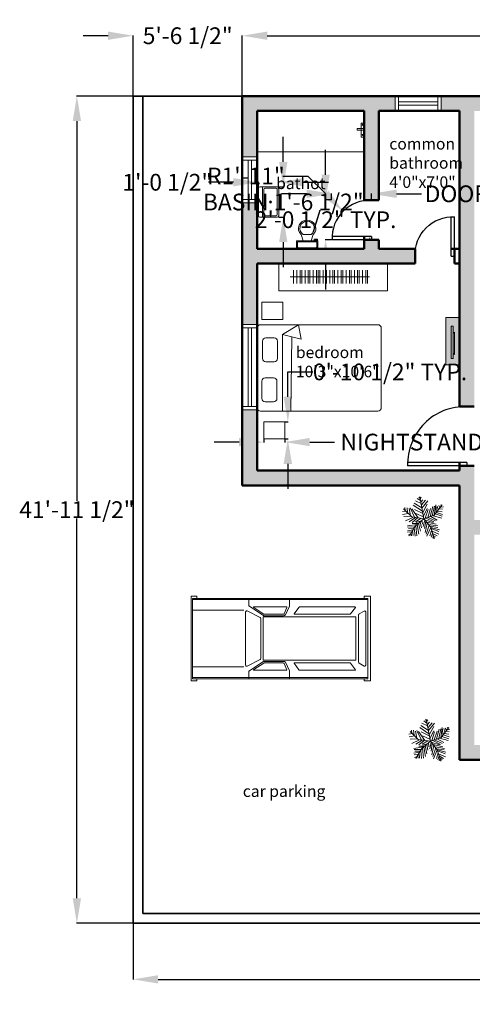
# Model space of a CAD drawing. Units: inches. Extents: x -2 to 7298, y -2 to 4583.
# Tile 1 of 6: x 5977 to 6252, y 3545 to 4144. Entities that reach past the tile are written whole.
import ezdxf

# ---------------------------------------------------------------- set-up
doc = ezdxf.new("R2010")
doc.units = ezdxf.units.IN
doc.header["$MEASUREMENT"] = 0
for name, color, linetype, lineweight in [('A-ANNO-DIMS', 2, 'Continuous', 18), ('A-AREA-IDEN', 7, 'Continuous', 18), ('A-DOOR', 4, 'Continuous', 25), ('A-FLOR-CASE', 30, 'Continuous', 18), ('A-FLOR-FIXT', 9, 'Continuous', 18), ('A-FURN', 8, 'Continuous', 18), ('A-FURN-PATT', 18, 'Continuous', 13), ('A-GLAZ', 4, 'Continuous', 18), ('A-SITE-VEHI', 51, 'Continuous', 18), ('A-WALL', 7, 'Continuous', 50), ('A-WALL-PATT', 18, 'Continuous', 13), ('C-PROP', 7, 'Continuous', 35), ('L-PLNT', 3, 'Continuous', 13)]:
    doc.layers.add(name, color=color, linetype=linetype, lineweight=lineweight)
doc.styles.get("Standard").update_dxf_attribs({"font": 'arial.ttf'})
doc.dimstyles.get("Standard").update_dxf_attribs({"dimtxt": 10.18, "dimasz": 15.18, "dimexe": 0.18, "dimexo": 0.0625, "dimgap": 0.09, "dimtad": 0, "dimtih": 1, "dimtoh": 1, "dimdec": 0, "dimzin": 0, "dimdsep": 46, "dimlunit": 3, "dimtxsty": 'Standard', "dimcen": 0.09, "dimadec": 0, "dimazin": 0, "dimtfac": 1, "dimtdec": 0, "dimtofl": 0, "dimtmove": 0, "dimatfit": 3, "dimfxl": 1, "dimtolj": 1, "dimtzin": 0, "dimarcsym": 0})

# ---------------------------------------------------------------- blocks, each defined once
blk = doc.blocks.new('*U4')
for p, q in [((-10, -8.5), (-8, -8.5)), ((-10, -9.5), (-10, -8.5)), ((-7, -9.5), (-10, -9.5)), ((-8, -8.5), (-8, -8)), ((-7, -8), (-7, -9.5)), ((-4, -8), (-6, -14)), ((4, -8), (6, -14)), ((9.5, -6), (9.5, -2)), ((4, -14), (-4, -14))]:
    blk.add_line(p, q)
blk.add_lwpolyline([(10.5, -8), (10.5, 0), (-10.5, 0), (-10.5, -8)], close=True)
for points in [[(-9.5, -2), (-9.5, -6)], [(8.5, -1), (-8.5, -1)], [(-8.5, -7), (8.5, -7)]]:
    blk.add_lwpolyline(points)
for centre, radius, start, end in [((-8.625, -1.875), 0.8839, 81.8699, 188.1301), ((-8.625, -6.125), 0.8839, 171.869898, 278.1301), ((8.625, -1.875), 0.8839, 351.8699, 98.1301), ((8.625, -6.125), 0.8839, 261.8699, 8.1301), ((-0.4772, -19.9188), 8.0953, 133.01722, 273.38), ((0.0374, -19.8731), 7.127, 124.50543, 269.7), ((-0.0373, -19.8731), 7.127, 270.3, 55.4946), ((0.4773, -19.9188), 8.0953, 266.62, 46.9828)]:
    blk.add_arc(centre, radius, start, end)
blk = doc.blocks.new('Sink-single - 30 in top')
blk.add_line((-15, -3.999996), (15, -3.999996))
for points in [[(-13.5, 0), (13.5, 0)], [(-15, -18.499996), (-15, -1.5)], [(-13.5, -17.499996), (-13.5, -6.499996)], [(-12.5, -5.499996), (12.5, -5.499996)], [(13.5, -6.499996), (13.5, -17.499996)], [(15, -1.5), (15, -18.499996)], [(12.5, -18.499996), (-12.5, -18.499996)], [(13.5, -19.999996), (-13.5, -19.999996)]]:
    blk.add_lwpolyline(points)
for radius in [1, 0.5]:
    blk.add_circle((0, -11.999996), radius)
for centre, radius, start, end in [((-13.5, -1.5), 1.5, 90, 180), ((-12.5, -6.499996), 1, 90, 180), ((12.5, -6.499996), 1, 0, 90), ((13.5, -1.5), 1.5, 0, 90), ((-13.5, -18.499996), 1.5, 180, 270), ((-12.5, -17.499996), 1, 180, 270), ((12.5, -17.499996), 1, 270, 0), ((13.5, -18.499996), 1.5, 270, 0)]:
    blk.add_arc(centre, radius, start, end)
blk = doc.blocks.new('*U9')
for p, q in [((32, 987), (4462, 987)), ((32, 715), (1324, 715)), ((32, -715), (1324, -715)), ((32, -987), (4462, -987))]:
    blk.add_line(p, q)
for points in [[(141, 1016), (141, 1071), (0, 1071), (0, -1071), (141, -1071), (141, -1016), (32, -1016), (32, 1016)], [(32, 1016), (4462, 1016), (4462, -1016), (32, -1016)], [(4362, 1016), (4462, 1016), (4462, -1016), (4362, -1016), (4362, -1071), (4525, -1071), (4525, 1071), (4362, 1071)], [(1815, 546), (4151, 546), (4151, -546), (1815, -546)]]:
    blk.add_lwpolyline(points, close=True)
for points in [[(1451, 1016), (1451, 823), (1822, 580, 0.086577), (1843, 576), (2326, 576, 0.227875), (2376, 600), (2482, 816), (2482, 1016)], [(1451, -1016), (1451, -823), (1822, -580, -0.086577), (1843, -576), (2326, -576, -0.227875), (2376, -600), (2482, -816), (2482, -1016)]]:
    blk.add_lwpolyline(points, format="xyb")
for points in [[(1577, 786), (1832, 618, 0.146139), (1846, 614), (2322, 614, 0.29766), (2345, 629), (2415, 789, 0.541236), (2409, 798), (1580, 798, 0.744989)], [(2596, 624), (2717, 787, -0.236929), (2737, 798), (4138, 798, -0.621576), (4143, 787), (4018, 624, -0.233368), (3998, 614), (2601, 614, -0.616908)], [(1410, 697), (1742, 531, -0.284287), (1756, 508), (1756, -508, -0.284287), (1742, -531), (1410, -697, -0.557284), (1373, -674), (1373, 674, -0.557284)], [(4366, 694), (4237, 622, 0.271143), (4224, 599), (4224, -599, 0.271143), (4237, -622), (4366, -694, 0.573387), (4404, -672), (4404, 672, 0.573387)], [(1577, -786), (1832, -618, -0.146139), (1846, -614), (2322, -614, -0.29766), (2345, -629), (2415, -789, -0.541236), (2409, -798), (1580, -798, -0.744989)], [(2596, -624), (2717, -787, 0.236929), (2737, -798), (4138, -798, 0.621576), (4143, -787), (4018, -624, 0.233368), (3998, -614), (2601, -614, 0.616908)]]:
    blk.add_lwpolyline(points, format="xyb", close=True)
blk = doc.blocks.new('*U11')
for p, q in [((-8.737, 47.138), (-17.069, 52.711)), ((-10.186, 53.64), (-13.084, 55.962)), ((0, 0), (-10.5, 57)), ((-9.099, 51.782), (-6.563, 55.962)), ((-48.585, 21.131), (-49.309, 29.026)), ((-43.513, 28.561), (-42.427, 15.558)), ((-38.442, 26.239), (-34.819, 7.663)), ((-35.544, 28.097), (-24.314, 3.947)), ((-3.665, 19.273), (-27.574, 35.527)), ((-5.114, 28.097), (-24.676, 40.636)), ((-7.288, 39.707), (-21.778, 46.673)), ((-7.65, 43.423), (-2.578, 49.46)), ((-5.839, 35.992), (4.667, 48.067)), ((-5.114, 27.632), (10.463, 46.673)), ((-2.941, 16.486), (8.652, 37.85)), ((-1.129, 6.734), (9.014, 26.704)), ((10.101, 3.483), (17.708, 26.239)), ((16.259, 5.805), (23.142, 31.348)), ((22.055, 7.198), (27.489, 32.277)), ((27, 9), (48, 36)), ((27.127, 9.056), (31.112, 35.992)), ((31.836, 30.883), (32.561, 16.486)), ((35.096, 32.741), (37.27, 22.524)), ((38.719, 34.134), (41.979, 28.561)), ((40.53, 25.775), (48.862, 24.846)), ((43.791, 29.954), (51.036, 30.883)), ((44.153, 36.456), (45.239, 32.741)), ((-47.498, 19.737), (-55.83, 18.344)), ((-40.615, 13.7), (-55.105, 10.913)), ((-31.5, 4.5), (-52.5, 25.5)), ((-33.37, 6.269), (-52.207, 5.34)), ((-28.299, 3.483), (-47.86, -5.805)), ((-21.416, 3.018), (-38.079, -8.128)), ((0, 0), (-31.5, 4.5)), ((-14.533, 2.09), (-30.834, 25.31)), ((-15.982, 2.09), (-30.11, -9.521)), ((-24.314, 23.917), (-2.941, 13.7)), ((0, 0), (-22.5, -19.5)), ((-6.563, 1.161), (-21.416, -8.128)), ((-20.691, 13.7), (-1.129, 4.876)), ((0, 0), (27, 9)), ((0, 0), (18, -22.5)), ((3.942, 1.625), (11.187, 24.381)), ((6.478, 1.625), (26.04, -8.592)), ((11.187, 3.483), (30.749, -5.805)), ((18.07, 5.805), (35.096, -3.483)), ((24.229, 7.663), (46.688, 1.625)), ((29.662, 12.307), (48.137, 6.269)), ((33.285, 16.486), (48.862, 10.913)), ((36.183, 19.737), (48.137, 17.88)), ((-17.431, -15.094), (-42.789, -18.809)), ((-24.314, -21.596), (-42.427, -22.06)), ((-22.5, -19.5), (-37.5, -45)), ((-15.257, -12.772), (-30.11, -12.772)), ((-25.038, -23.918), (-22.865, -45.281)), ((-20.691, -18.345), (-17.793, -44.352)), ((-6.563, -5.805), (-19.967, -9.985)), ((-17.069, -15.094), (-12.721, -40.172)), ((-13.446, -11.378), (-8.737, -32.741)), ((-9.461, -8.592), (-6.201, -23.453)), ((-4.752, -3.483), (-3.665, -14.629)), ((2.493, -3.019), (-1.491, -20.202)), ((1.769, -2.555), (24.229, -9.521)), ((5.029, -6.27), (2.131, -25.775)), ((9.014, -11.378), (3.58, -35.992)), ((14.085, -16.951), (6.478, -40.172)), ((7.565, -9.056), (32.198, -14.629)), ((18.07, -22.524), (8.289, -45.745)), ((12.274, -15.094), (36.907, -18.809)), ((16.259, -19.738), (36.183, -22.989)), ((18, -22.5), (27, -52.5)), ((18.433, -22.524), (40.53, -29.026)), ((19.157, -25.311), (38.719, -33.206)), ((-28.299, -29.026), (-42.789, -31.348)), ((-30.834, -34.135), (-42.427, -35.528)), ((-34.457, -39.708), (-40.978, -42.494)), ((-26.849, -26.24), (-40.253, -25.775)), ((-32.646, -36.921), (-31.921, -44.352)), ((-29.023, -30.884), (-27.936, -43.887)), ((20.244, -30.419), (15.897, -44.816)), ((22.78, -37.85), (19.519, -48.532)), ((21.331, -32.741), (39.081, -40.636)), ((22.78, -38.314), (34.372, -44.816)), ((24.591, -45.745), (23.142, -50.854)), ((24.591, -43.423), (30.749, -47.603)), ((26.764, -49.925), (28.213, -50.854))]:
    blk.add_line(p, q)
blk = doc.blocks.new('WINDOW-48IN')
for p, q in [((-2, 4.5), (-2, -4.5)), ((0, 4.5), (0, -4.5)), ((0, 1), (48, 1)), ((48, 4.5), (48, -4.5)), ((50, 4.5), (50, -4.5)), ((0, -1), (48, -1))]:
    blk.add_line(p, q)
blk = doc.blocks.new('WINDOW-24IN')
for p, q in [((-26, 4.5), (-26, -4.5)), ((-24, 4.5), (-24, -4.5)), ((-24, 1), (0, 1)), ((0, 4.5), (0, -4.5)), ((2, 4.5), (2, -4.5)), ((-24, -1), (0, -1))]:
    blk.add_line(p, q)
blk = doc.blocks.new('DOOR-SWING-36IN')
for p, q in [((0, 0), (0, 36)), ((2, 0), (2, 36)), ((2, 0), (0, 0))]:
    blk.add_line(p, q)
blk.add_arc((1, 1), 35.01, 358.36342, 91.63658)
blk = doc.blocks.new('DOOR-SWING-24IN')
for p, q in [((0, 2), (-24, 2)), ((0, 2), (0, 0)), ((0, 0), (-24, 0))]:
    blk.add_line(p, q)
blk.add_arc((-1, 1), 23.02, 87.51045, 182.48955)
blk = doc.blocks.new('NIGHTSTAND-B')
blk.add_lwpolyline([(0, 10.48), (0, 10.48), (12.59, 10.48), (12.59, 10.48), (12.59, 0), (12.59, 0), (0, 0), (0, 0)], close=True)
blk = doc.blocks.new('*D43')
at = {"layer": 'A-ANNO-DIMS', "color": 0, "lineweight": -2, "transparency": 16777216}
for p, q in [((6151.67, 4038.42), (6136.49, 4038.42)), ((6166.85, 4034.84), (6166.85, 4038.6)), ((6191.14, 4034.84), (6191.14, 4038.6)), ((6206.32, 4038.42), (6221.5, 4038.42))]:
    blk.add_line(p, q, dxfattribs=at)
at = {"layer": 'A-ANNO-DIMS', "color": 0, "transparency": 16777216}
for points in [[(6151.67, 4040.95), (6151.67, 4035.89), (6166.85, 4038.42)], [(6206.32, 4040.95), (6206.32, 4035.89), (6191.14, 4038.42)]]:
    blk.add_solid(points, dxfattribs=at)
at = {"layer": 'Defpoints', "color": 0, "transparency": 16777216}
for p in [(6166.85, 4034.78), (6191.14, 4038.42), (6191.14, 4034.78)]:
    blk.add_point(p, dxfattribs=at)
at = {"layer": 'A-ANNO-DIMS', "color": 0, "transparency": 16777216, "insert": (6287.53, 4038.42), "char_height": 10.18, "attachment_point": 5}
blk.add_mtext('\\A1;DOOR 2\'-0 1/2" TYP.', dxfattribs=at)
blk = doc.blocks.new('*D44')
at = {"layer": 'A-ANNO-DIMS', "color": 0, "lineweight": -2, "transparency": 16777216}
for p, q in [((6163.21, 4049.96), (6163.21, 4065.14)), ((6166.79, 4034.78), (6163.03, 4034.78)), ((6166.79, 4010.49), (6163.03, 4010.49)), ((6163.21, 3995.31), (6163.21, 3980.13))]:
    blk.add_line(p, q, dxfattribs=at)
at = {"layer": 'A-ANNO-DIMS', "color": 0, "transparency": 16777216}
for points in [[(6160.68, 4049.96), (6165.74, 4049.96), (6163.21, 4034.78)], [(6160.68, 3995.31), (6165.74, 3995.31), (6163.21, 4010.49)]]:
    blk.add_solid(points, dxfattribs=at)
at = {"layer": 'Defpoints', "color": 0, "transparency": 16777216}
for p in [(6163.21, 4034.78), (6166.85, 4034.78), (6166.85, 4010.49)]:
    blk.add_point(p, dxfattribs=at)
at = {"layer": 'A-ANNO-DIMS', "color": 0, "transparency": 16777216, "insert": (6163.21, 4022.64), "char_height": 10.18, "attachment_point": 5}
blk.add_mtext('\\A1;2\'-0 1/2" TYP.', dxfattribs=at)
blk = doc.blocks.new('*D55')
at = {"layer": 'A-ANNO-DIMS', "color": 0, "lineweight": -2, "transparency": 16777216}
for p, q in [((6110.57, 3887.28), (6095.39, 3887.28)), ((6125.75, 3889.11), (6125.75, 3887.1)), ((6138.34, 3889.11), (6138.34, 3887.1)), ((6153.52, 3887.28), (6168.7, 3887.28))]:
    blk.add_line(p, q, dxfattribs=at)
at = {"layer": 'A-ANNO-DIMS', "color": 0, "transparency": 16777216}
for points in [[(6110.57, 3889.81), (6110.57, 3884.75), (6125.75, 3887.28)], [(6153.52, 3889.81), (6153.52, 3884.75), (6138.34, 3887.28)]]:
    blk.add_solid(points, dxfattribs=at)
at = {"layer": 'Defpoints', "color": 0, "transparency": 16777216}
for p in [(6125.75, 3889.17), (6138.34, 3889.17), (6138.34, 3887.28)]:
    blk.add_point(p, dxfattribs=at)
at = {"layer": 'A-ANNO-DIMS', "color": 0, "transparency": 16777216, "insert": (6266.35, 3887.28), "char_height": 10.18, "attachment_point": 5}
blk.add_mtext('\\A1;NIGHTSTAND B 1\'-0 1/2" TYP.', dxfattribs=at)
blk = doc.blocks.new('*D56')
at = {"layer": 'A-ANNO-DIMS', "color": 0, "lineweight": -2, "transparency": 16777216}
for p, q in [((6140.23, 3914.83), (6140.23, 3930.01)), ((6140.23, 3930.01), (6155.41, 3930.01)), ((6138.4, 3899.65), (6140.41, 3899.65)), ((6138.4, 3889.17), (6140.41, 3889.17)), ((6140.23, 3873.99), (6140.23, 3858.81))]:
    blk.add_line(p, q, dxfattribs=at)
at = {"layer": 'A-ANNO-DIMS', "color": 0, "transparency": 16777216}
for points in [[(6137.7, 3914.83), (6142.76, 3914.83), (6140.23, 3899.65)], [(6137.7, 3873.99), (6142.76, 3873.99), (6140.23, 3889.17)]]:
    blk.add_solid(points, dxfattribs=at)
at = {"layer": 'Defpoints', "color": 0, "transparency": 16777216}
for p in [(6138.34, 3899.65), (6140.23, 3899.65), (6138.34, 3889.17)]:
    blk.add_point(p, dxfattribs=at)
at = {"layer": 'A-ANNO-DIMS', "color": 0, "transparency": 16777216, "insert": (6202.34, 3930.01), "char_height": 10.18, "attachment_point": 5}
blk.add_mtext('\\A1;0\'-10 1/2" TYP.', dxfattribs=at)
blk = doc.blocks.new('*D59')
at = {"layer": 'A-ANNO-DIMS', "color": 0, "lineweight": -2, "transparency": 16777216}
for p, q in [((6137.45, 4057.85), (6137.45, 4073.03)), ((6134.74, 4042.67), (6137.63, 4042.67)), ((6134.74, 4024.18), (6137.63, 4024.18)), ((6137.45, 4009), (6137.45, 3993.82))]:
    blk.add_line(p, q, dxfattribs=at)
at = {"layer": 'A-ANNO-DIMS', "color": 0, "transparency": 16777216}
for points in [[(6134.92, 4057.85), (6139.98, 4057.85), (6137.45, 4042.67)], [(6134.92, 4009), (6139.98, 4009), (6137.45, 4024.18)]]:
    blk.add_solid(points, dxfattribs=at)
at = {"layer": 'Defpoints', "color": 0, "transparency": 16777216}
for p in [(6134.67, 4042.67), (6137.45, 4042.67), (6134.67, 4024.18)]:
    blk.add_point(p, dxfattribs=at)
at = {"layer": 'A-ANNO-DIMS', "color": 0, "transparency": 16777216, "insert": (6137.45, 4033.42), "char_height": 10.18, "attachment_point": 5}
blk.add_mtext('\\A1;BASIN 1\'-6 1/2"', dxfattribs=at)
blk = doc.blocks.new('*D60')
at = {"layer": 'A-ANNO-DIMS', "color": 0, "lineweight": -2, "transparency": 16777216}
for p, q in [((6122.34, 4042.74), (6122.34, 4045.63)), ((6134.67, 4042.74), (6134.67, 4045.63)), ((6107.16, 4045.45), (6091.98, 4045.45)), ((6149.85, 4045.45), (6165.03, 4045.45))]:
    blk.add_line(p, q, dxfattribs=at)
at = {"layer": 'A-ANNO-DIMS', "color": 0, "transparency": 16777216}
for points in [[(6107.16, 4047.98), (6107.16, 4042.92), (6122.34, 4045.45)], [(6149.85, 4047.98), (6149.85, 4042.92), (6134.67, 4045.45)]]:
    blk.add_solid(points, dxfattribs=at)
at = {"layer": 'Defpoints', "color": 0, "transparency": 16777216}
for p in [(6122.34, 4045.45), (6122.34, 4042.67), (6134.67, 4042.67)]:
    blk.add_point(p, dxfattribs=at)
at = {"layer": 'A-ANNO-DIMS', "color": 0, "transparency": 16777216, "insert": (6066.98, 4045.45), "char_height": 10.18, "attachment_point": 5}
blk.add_mtext('\\A1;1\'-0 1/2"', dxfattribs=at)
blk = doc.blocks.new('*D61')
at = {"layer": 'A-ANNO-DIMS', "color": 0, "lineweight": -2, "transparency": 16777216}
for p, q in [((6046.17, 3594.33), (6046.17, 3560.06)), ((6720.58, 3594.33), (6720.58, 3560.06)), ((6061.35, 3560.24), (6353.94, 3560.24)), ((6705.4, 3560.24), (6412.81, 3560.24))]:
    blk.add_line(p, q, dxfattribs=at)
at = {"layer": 'A-ANNO-DIMS', "color": 0, "transparency": 16777216}
for points in [[(6061.35, 3562.77), (6061.35, 3557.71), (6046.17, 3560.24)], [(6705.4, 3562.77), (6705.4, 3557.71), (6720.58, 3560.24)]]:
    blk.add_solid(points, dxfattribs=at)
at = {"layer": 'Defpoints', "color": 0, "transparency": 16777216}
for p in [(6046.17, 3594.39), (6720.58, 3594.39), (6720.58, 3560.24)]:
    blk.add_point(p, dxfattribs=at)
at = {"layer": 'A-ANNO-DIMS', "color": 0, "transparency": 16777216, "insert": (6383.37, 3560.24), "char_height": 10.18, "attachment_point": 5}
blk.add_mtext('\\A1;56\'-2 1/2"', dxfattribs=at)
blk = doc.blocks.new('*D62')
at = {"layer": 'A-ANNO-DIMS', "color": 0, "lineweight": -2, "transparency": 16777216}
for p, q in [((6046.1, 4097.9), (6011.84, 4097.9)), ((6012.02, 4082.72), (6012.02, 3851.5)), ((6012.02, 3609.57), (6012.02, 3840.79)), ((6046.1, 3594.39), (6011.84, 3594.39))]:
    blk.add_line(p, q, dxfattribs=at)
at = {"layer": 'A-ANNO-DIMS', "color": 0, "transparency": 16777216}
for points in [[(6009.49, 4082.72), (6014.55, 4082.72), (6012.02, 4097.9)], [(6009.49, 3609.57), (6014.55, 3609.57), (6012.02, 3594.39)]]:
    blk.add_solid(points, dxfattribs=at)
at = {"layer": 'Defpoints', "color": 0, "transparency": 16777216}
for p in [(6012.02, 4097.9), (6046.17, 4097.9), (6046.17, 3594.39)]:
    blk.add_point(p, dxfattribs=at)
at = {"layer": 'A-ANNO-DIMS', "color": 0, "transparency": 16777216, "insert": (6012.02, 3846.15), "char_height": 10.18, "attachment_point": 5}
blk.add_mtext('\\A1;41\'-11 1/2"', dxfattribs=at)
blk = doc.blocks.new('*D64')
at = {"layer": 'A-ANNO-DIMS', "color": 0, "lineweight": -2, "transparency": 16777216}
for p, q in [((6112.58, 4097.97), (6112.58, 4134.81)), ((6127.76, 4134.63), (6399, 4134.63)), ((6705.4, 4134.63), (6434.15, 4134.63)), ((6720.58, 4097.97), (6720.58, 4134.81))]:
    blk.add_line(p, q, dxfattribs=at)
at = {"layer": 'A-ANNO-DIMS', "color": 0, "transparency": 16777216}
for points in [[(6127.76, 4137.16), (6127.76, 4132.1), (6112.58, 4134.63)], [(6705.4, 4137.16), (6705.4, 4132.1), (6720.58, 4134.63)]]:
    blk.add_solid(points, dxfattribs=at)
at = {"layer": 'Defpoints', "color": 0, "transparency": 16777216}
for p in [(6720.58, 4134.63), (6112.58, 4097.9), (6720.58, 4097.9)]:
    blk.add_point(p, dxfattribs=at)
at = {"layer": 'A-ANNO-DIMS', "color": 0, "transparency": 16777216, "insert": (6416.58, 4134.63), "char_height": 10.18, "attachment_point": 5}
blk.add_mtext('\\A1;50\'-8"', dxfattribs=at)
blk = doc.blocks.new('*D66')
at = {"layer": 'A-ANNO-DIMS', "color": 0, "lineweight": -2, "transparency": 16777216}
for p, q in [((6030.986562, 4134.626544), (6015.806562, 4134.626544)), ((6046.166562, 4097.966533), (6046.166562, 4134.806544)), ((6112.578072, 4097.966533), (6112.578072, 4134.806544)), ((6127.758072, 4134.626544), (6142.938072, 4134.626544))]:
    blk.add_line(p, q, dxfattribs=at)
at = {"layer": 'A-ANNO-DIMS', "color": 0, "transparency": 16777216}
for points in [[(6030.986562, 4137.156544), (6030.986562, 4132.096544), (6046.166562, 4134.626544)], [(6127.758072, 4137.156544), (6127.758072, 4132.096544), (6112.578072, 4134.626544)]]:
    blk.add_solid(points, dxfattribs=at)
at = {"layer": 'Defpoints', "color": 0, "transparency": 16777216}
for p in [(6112.578072, 4134.626544), (6046.166562, 4097.904033), (6112.578072, 4097.904033)]:
    blk.add_point(p, dxfattribs=at)
at = {"layer": 'A-ANNO-DIMS', "color": 0, "transparency": 16777216, "insert": (6079.372317, 4134.626544), "char_height": 10.18, "attachment_point": 5}
blk.add_mtext('\\A1;5\'-6 1/2"', dxfattribs=at)
blk = doc.blocks.new('*D94')
at = {"layer": 'A-ANNO-DIMS', "color": 0, "lineweight": -2, "transparency": 16777216}
for p, q in [((6137.21, 4049.24), (6152.39, 4049.24)), ((6152.39, 4049.24), (6163.12, 4038.51)), ((6190.05, 4011.49), (6190.23, 4011.49)), ((6190.14, 4011.4), (6190.14, 4011.58))]:
    blk.add_line(p, q, dxfattribs=at)
at = {"layer": 'A-ANNO-DIMS', "color": 0, "transparency": 16777216}
blk.add_solid([(6164.91, 4040.3), (6161.33, 4036.72), (6173.86, 4027.77)], dxfattribs=at)
at = {"layer": 'Defpoints', "color": 0, "transparency": 16777216}
for p in [(6173.86, 4027.77), (6190.14, 4011.49)]:
    blk.add_point(p, dxfattribs=at)
at = {"layer": 'A-ANNO-DIMS', "color": 0, "transparency": 16777216, "insert": (6114.76, 4049.24), "char_height": 10.18, "attachment_point": 5}
blk.add_mtext('\\A1;R1\'-11"', dxfattribs=at)

msp = doc.modelspace()

# ---------------------------------------------------------------- hatches: boundary and pattern name
at = {"layer": 'A-FURN-PATT'}
h = msp.add_hatch(color=256, dxfattribs=at)
h.dxf.hatch_style = 1
h.paths.add_polyline_path([(6244.58, 3963.09), (6236.19, 3963.09), (6236.19, 3934.4), (6244.58, 3934.4)])
at = {"layer": 'A-WALL-PATT'}
h = msp.add_hatch(color=256, dxfattribs=at)
h.dxf.hatch_style = 1
h.paths.add_polyline_path([(6253.58, 3872.9), (6244.58, 3872.9), (6244.58, 3869.9), (6121.58, 3869.9), (6121.58, 3906.9), (6112.58, 3906.9), (6112.58, 3860.9), (6244.58, 3860.9), (6244.58, 3693.9), (6289.08, 3693.9), (6289.08, 3702.9), (6253.58, 3702.9), (6253.58, 3830.9), (6337.58, 3830.9), (6337.58, 3833.4, -0.014283), (6337.58, 3835.4), (6337.58, 3839.9), (6253.58, 3839.9)])
h.paths.add_polyline_path([(6385.58, 3839.9), (6373.58, 3839.9), (6373.58, 3830.9), (6376.58, 3830.9), (6376.58, 3702.9), (6341.08, 3702.9), (6341.08, 3693.9), (6410.08, 3693.9), (6410.08, 3702.9), (6385.58, 3702.9)])
h.paths.add_polyline_path([(6519.58, 3864.9), (6557.19, 3864.9), (6557.19, 3873.9), (6510.58, 3873.9), (6510.58, 3839.9), (6510.58, 3702.9), (6486.08, 3702.9), (6486.08, 3693.9), (6562.53, 3693.9), (6562.53, 3702.9), (6519.58, 3702.9)])
h.paths.add_polyline_path([(6666.47, 3745.9), (6657.47, 3745.9), (6657.47, 3702.9), (6614.53, 3702.9), (6614.53, 3693.9), (6666.47, 3693.9)])
h.paths.add_polyline_path([(6666.47, 3926.97), (6661.97, 3926.97, -0.014283), (6659.97, 3926.97), (6657.47, 3926.97), (6657.47, 3873.9), (6606.04, 3873.9), (6606.04, 3864.9), (6657.47, 3864.9), (6657.47, 3821.9), (6666.47, 3821.9)])
h.paths.add_polyline_path([(6720.58, 4097.9), (6547.84, 4097.9), (6547.84, 4088.9), (6606.58, 4088.9), (6606.58, 3997.9, 0.414214), (6608.58, 3995.9), (6618.58, 3995.9), (6618.58, 4004.9), (6615.58, 4004.9), (6615.58, 4088.9), (6711.58, 4088.9), (6711.58, 4060.9), (6720.58, 4060.9)])
h.paths.add_polyline_path([(6720.58, 4032.9), (6711.58, 4032.9), (6711.58, 4004.9), (6654.58, 4004.9), (6654.58, 4002.4, -0.014283), (6654.58, 4000.4), (6654.58, 3995.9), (6711.58, 3995.9), (6720.58, 3995.9)], flags=17)
h.paths.add_polyline_path([(6471.84, 4097.9), (6233.45, 4097.9), (6233.45, 4088.9), (6244.58, 4088.9), (6244.58, 4004.9), (6244.58, 3995.9), (6244.58, 3908.9), (6247.08, 3908.9, -0.014283), (6249.08, 3908.9), (6253.58, 3908.9), (6253.58, 3995.9), (6253.58, 4088.9), (6392.58, 4088.9), (6392.58, 4004.9), (6392.58, 3995.9), (6392.58, 3894.9), (6401.58, 3894.9), (6401.58, 3995.9), (6401.58, 4004.9), (6401.58, 4088.9), (6471.84, 4088.9)])
h.paths.add_polyline_path([(6205.45, 4097.9), (6112.58, 4097.9), (6112.58, 4060.9), (6121.58, 4060.9), (6121.58, 4088.9), (6186.64, 4088.9), (6186.64, 4034.49), (6189.14, 4034.49, -0.021729), (6191.14, 4034.49), (6195.64, 4034.49), (6195.64, 4088.9), (6202.58, 4088.9), (6205.45, 4088.9)])
h.paths.add_polyline_path([(6121.58, 3995.9), (6217.58, 3995.9), (6217.58, 4000.4, -0.021729), (6217.58, 4002.4), (6217.58, 4004.9), (6195.64, 4004.9), (6195.64, 4010.49), (6186.64, 4010.49), (6186.64, 4004.9), (6121.58, 4004.9), (6121.58, 4032.9), (6112.58, 4032.9), (6112.58, 3958.9), (6121.58, 3958.9)])

# ---------------------------------------------------------------- linework, layer by layer
at = {"layer": 'A-FLOR-CASE'}
for p, q in [((6134.73, 3995.9), (6134.73, 3979.41)), ((6143.69, 3992.01), (6143.69, 3983.76)), ((6145.69, 3992.01), (6145.69, 3983.76)), ((6147.69, 3992.01), (6147.69, 3983.76)), ((6148.69, 3992.01), (6148.69, 3983.76)), ((6150.69, 3992.01), (6150.69, 3983.76)), ((6152.69, 3992.01), (6152.69, 3983.76)), ((6153.69, 3992.01), (6153.69, 3983.76)), ((6155.69, 3992.01), (6155.69, 3983.76)), ((6157.69, 3992.01), (6157.69, 3983.76)), ((6157.69, 3992.01), (6157.69, 3983.76)), ((6157.69, 3992.01), (6157.69, 3983.76)), ((6158.69, 3992.01), (6158.69, 3983.76)), ((6159.69, 3992.01), (6159.69, 3983.76)), ((6159.69, 3992.01), (6159.69, 3983.76)), ((6161.69, 3992.01), (6161.69, 3983.76)), ((6163.69, 3992.01), (6163.69, 3983.76)), ((6163.69, 3992.01), (6163.69, 3983.76)), ((6165.69, 3992.01), (6165.69, 3983.76)), ((6167.69, 3992.01), (6167.69, 3983.76)), ((6168.69, 3992.01), (6168.69, 3983.76)), ((6170.69, 3992.01), (6170.69, 3983.76)), ((6172.69, 3992.01), (6172.69, 3983.76)), ((6173.69, 3992.01), (6173.69, 3983.76)), ((6175.69, 3992.01), (6175.69, 3983.76)), ((6177.69, 3992.01), (6177.69, 3983.76)), ((6178.69, 3992.01), (6178.69, 3983.76)), ((6180.69, 3992.01), (6180.69, 3983.76)), ((6182.69, 3992.01), (6182.69, 3983.76)), ((6183.69, 3992.01), (6183.69, 3983.76)), ((6185.69, 3992.01), (6185.69, 3983.76)), ((6187.69, 3992.01), (6187.69, 3983.76)), ((6188.69, 3992.01), (6188.69, 3983.76)), ((6200.82, 3979.41), (6200.82, 3995.9)), ((6141.7, 3987.87), (6189.79, 3987.87)), ((6134.73, 3979.41), (6200.82, 3979.41))]:
    msp.add_line(p, q, dxfattribs=at)
at = {"layer": 'A-FLOR-FIXT'}
for p, q in [((6182.35, 4077.17), (6182.35, 4078.15)), ((6182.35, 4078.15), (6186.64, 4078.15)), ((6186.64, 4077.17), (6182.35, 4077.17)), ((6121.58, 4064.05), (6186.64, 4064.05))]:
    msp.add_line(p, q, dxfattribs=at)
msp.add_lwpolyline([(6186.64, 4081.43), (6186.64, 4081.43), (6184.91, 4081.43), (6184.91, 4081.43), (6184.91, 4072.91), (6184.91, 4072.91), (6186.64, 4072.91), (6186.64, 4072.91)], close=True, dxfattribs=at)
for centre in [(6185.8, 4080.39), (6185.8, 4074.21)]:
    msp.add_circle(centre, 0.369, dxfattribs=at)
at = {"layer": 'A-FURN'}
for p, q in [((6136.95, 3952.68), (6146.68, 3958.73)), ((6146.68, 3958.73), (6148.41, 3949.98)), ((6137.06, 3906.2), (6136.95, 3952.68)), ((6148.41, 3949.98), (6136.95, 3952.68)), ((6142.09, 3906.2), (6142.68, 3951.33)), ((6240.76, 3953.65), (6241.54, 3954.11)), ((6241.54, 3954.11), (6241.54, 3940.63)), ((6241.54, 3940.63), (6240.76, 3941.42))]:
    msp.add_line(p, q, dxfattribs=at)
for points in [[(6244.58, 3963.09), (6244.58, 3963.09), (6236.19, 3963.09), (6236.19, 3963.09), (6236.19, 3934.4), (6236.19, 3934.4), (6244.58, 3934.4), (6244.58, 3934.4)], [(6240.76, 3957.77), (6240.76, 3957.77), (6239.58, 3957.77), (6239.58, 3957.77), (6239.58, 3938.17), (6239.58, 3938.17), (6240.76, 3938.17), (6240.76, 3938.17)]]:
    msp.add_lwpolyline(points, close=True, dxfattribs=at)
for points in [[(6121.58, 3956.73, -0.414214), (6123.58, 3958.73), (6195.05, 3958.73, -0.414214), (6197.05, 3956.73), (6197.05, 3908.2, -0.414214), (6195.05, 3906.2), (6123.58, 3906.2, -0.414214), (6121.58, 3908.2)], [(6124.83, 3938.17, 0.414214), (6126.83, 3936.17), (6131.95, 3936.17, 0.414214), (6133.95, 3938.17), (6133.95, 3948.7, 0.414214), (6131.95, 3950.7), (6126.83, 3950.7, 0.414214), (6124.83, 3948.7)], [(6124.49, 3913.79, 0.414214), (6126.49, 3911.79), (6131.61, 3911.79, 0.414214), (6133.61, 3913.79), (6133.61, 3924.32, 0.414214), (6131.61, 3926.32), (6126.49, 3926.32, 0.414214), (6124.49, 3924.32)]]:
    msp.add_lwpolyline(points, format="xyb", close=True, dxfattribs=at)
at = {"layer": 'A-WALL'}
for p, q in [((6112.58, 3860.9), (6112.58, 4097.9)), ((6112.58, 4097.9), (6720.58, 4097.9)), ((6121.58, 4088.9), (6186.64, 4088.9)), ((6121.58, 4004.9), (6121.58, 4088.9)), ((6186.64, 4088.9), (6186.64, 4034.25)), ((6195.64, 4088.9), (6195.64, 4034.49)), ((6195.64, 4088.9), (6202.58, 4088.9)), ((6202.58, 4088.9), (6211.58, 4088.9)), ((6211.58, 4088.9), (6244.58, 4088.9)), ((6244.58, 4004.9), (6244.58, 4088.9)), ((6186.64, 4034.49), (6195.64, 4034.49)), ((6186.64, 4012.49), (6186.64, 4004.9)), ((6186.64, 4010.49), (6195.64, 4010.49)), ((6195.64, 4010.49), (6195.64, 4004.9)), ((6121.58, 4004.9), (6186.64, 4004.9)), ((6195.64, 4004.9), (6217.82, 4004.9)), ((6217.58, 4004.9), (6217.58, 3995.9)), ((6239.58, 4004.9), (6244.58, 4004.9)), ((6241.58, 4004.9), (6241.58, 3995.9)), ((6244.58, 4004.9), (6244.58, 3995.9)), ((6121.58, 3869.9), (6121.58, 3995.9)), ((6121.58, 3995.9), (6217.58, 3995.9)), ((6241.58, 3995.9), (6244.58, 3995.9)), ((6244.58, 3908.74), (6244.58, 3995.9)), ((6244.58, 3908.9), (6253.58, 3908.9)), ((6244.58, 3869.9), (6244.58, 3874.9)), ((6244.58, 3872.9), (6253.58, 3872.9)), ((6121.58, 3869.9), (6244.58, 3869.9)), ((6112.58, 3860.9), (6244.58, 3860.9)), ((6244.58, 3693.9), (6244.58, 3860.9)), ((6666.47, 3693.9), (6244.58, 3693.9))]:
    msp.add_line(p, q, dxfattribs=at)
at = {"layer": 'C-PROP'}
for p, q in [((6046.17, 3594.39), (6046.17, 4097.9)), ((6046.17, 4097.9), (6112.58, 4097.9)), ((6052.17, 3600.39), (6052.17, 4097.9)), ((6714.58, 3600.39), (6052.17, 3600.39)), ((6720.58, 3594.39), (6046.17, 3594.39))]:
    msp.add_line(p, q, dxfattribs=at)

# ---------------------------------------------------------------- block references
at = {"layer": 'A-DOOR'}
msp.add_blockref('DOOR-SWING-24IN', (6191.14, 4010.49), dxfattribs=at)
at = {"layer": 'A-DOOR', "extrusion": (0, 0, -1), "zscale": -1, "rotation": 269.9999999999921}
msp.add_blockref('DOOR-SWING-24IN', (-6241.58, 4000.4), dxfattribs=at)
at = {"layer": 'A-DOOR', "rotation": 90.0000000000023}
msp.add_blockref('DOOR-SWING-36IN', (6249.08, 3872.9), dxfattribs=at)
at = {"layer": 'A-FLOR-FIXT'}
for name, p, xscale, yscale, zscale, rotation in [('Sink-single - 30 in top', (6122.34, 4033.42), 0.6166051231948902, 0.6166051231948902, 0.6166051231948902, 90), ('*U4', (6151.98, 4004.9), 0.6219973566643829, 0.6219973566643829, 0.6219973566643829, 180)]:
    msp.add_blockref(name, p, dxfattribs=dict(at, xscale=xscale, yscale=yscale, zscale=zscale, rotation=rotation))
at = {"layer": 'A-FURN'}
for p in [(6124.54, 3961.95), (6125.75, 3889.17)]:
    msp.add_blockref('NIGHTSTAND-B', p, dxfattribs=at)
at = {"layer": 'A-GLAZ'}
msp.add_blockref('WINDOW-24IN', (6231.45, 4093.4), dxfattribs=at)
for name, p, rotation in [('WINDOW-24IN', (6117.08, 4034.9), 270.0000000000078), ('WINDOW-48IN', (6117.08, 3956.9), 270.0000000000056)]:
    msp.add_blockref(name, p, dxfattribs=dict(at, rotation=rotation))
at = {"layer": 'A-SITE-VEHI', "xscale": 0.0240846404363074, "yscale": 0.0240846404363074, "zscale": 0.0240846404363074}
msp.add_blockref('*U9', (6081.51, 3767.69), dxfattribs=at)
at = {"layer": 'L-PLNT', "xscale": 0.2336039447018575, "yscale": 0.2336039447018575, "zscale": 0.2336039447018575}
for p in [(6222.9, 3840.65), (6226.88, 3705.23)]:
    msp.add_blockref('*U11', p, dxfattribs=at)

# ---------------------------------------------------------------- texts
at = {"layer": 'A-AREA-IDEN', "char_height": 7, "attachment_point": 1}
for s, insert in [('common\\Pbathroom\\P4\'0"x7\'0"', (6201.93, 4072.36)), ('bathot', (6133.13, 4048.25)), ('bedroom\\P10\'3"x10\'6"', (6145.13, 3945.41)), ('car parking', (6112.86, 3678.29))]:
    msp.add_mtext_dynamic_manual_height_columns(s, width=127.1277, gutter_width=1, heights=[0], dxfattribs=dict(at, insert=insert))

# ---------------------------------------------------------------- dimensions: what is measured, and where the dimension line sits
at = {"layer": 'A-ANNO-DIMS'}
for base, p1, p2, picture, middle in [((6112.58, 4134.63), (6046.17, 4097.9), (6112.58, 4097.9), '*D66', (6079.37, 4134.63)), ((6720.58, 4134.63), (6112.58, 4097.9), (6720.58, 4097.9), '*D64', (6416.58, 4134.63)), ((6720.58, 3560.24), (6046.17, 3594.39), (6720.58, 3594.39), '*D61', (6383.37, 3560.24))]:
    dim = msp.add_linear_dim(base=base, p1=p1, p2=p2, dimstyle='Standard', override={"dimdec": 1, "dimlfac": 1, "dimrnd": 0, "dimzin": 1, "dimdsep": 46, "dimlunit": 4, "dimfrac": 2}, dxfattribs=at)
    dim.commit()
    dim.dimension.update_dxf_attribs({"geometry": picture, "text_midpoint": middle})
for base, p1, p2, angle, picture, middle in [((6012.02, 4097.9), (6046.17, 3594.39), (6046.17, 4097.9), 90, '*D62', (6012.02, 3846.15)), ((6122.34, 4045.45), (6134.67, 4042.67), (6122.34, 4042.67), 180, '*D60', (6066.98, 4045.45))]:
    dim = msp.add_linear_dim(base=base, p1=p1, p2=p2, angle=angle, dimstyle='Standard', override={"dimdec": 1, "dimlfac": 1, "dimrnd": 0, "dimzin": 1, "dimdsep": 46, "dimlunit": 4, "dimfrac": 2}, dxfattribs=at)
    dim.commit()
    dim.dimension.update_dxf_attribs({"geometry": picture, "text_midpoint": middle})
for base, p1, p2, text, picture, middle in [((6137.45, 4042.67), (6134.67, 4024.18), (6134.67, 4042.67), 'BASIN <>', '*D59', (6137.45, 4033.42)), ((6163.21, 4034.78), (6166.85, 4010.49), (6166.85, 4034.78), '<> TYP.', '*D44', (6163.21, 4022.64)), ((6140.23, 3899.65), (6138.34, 3889.17), (6138.34, 3899.65), '<> TYP.', '*D56', (6202.34, 3930.01))]:
    dim = msp.add_linear_dim(base=base, p1=p1, p2=p2, angle=90, text=text, dimstyle='Standard', override={"dimdec": 1, "dimlfac": 1, "dimrnd": 0, "dimzin": 1, "dimdsep": 46, "dimlunit": 4, "dimfrac": 2}, dxfattribs=at)
    dim.commit()
    dim.dimension.update_dxf_attribs({"geometry": picture, "text_midpoint": middle})
for base, p1, p2, text, picture, middle in [((6191.14, 4038.42), (6166.85, 4034.78), (6191.14, 4034.78), 'DOOR <> TYP.', '*D43', (6287.53, 4038.42)), ((6138.34, 3887.28), (6125.75, 3889.17), (6138.34, 3889.17), 'NIGHTSTAND B <> TYP.', '*D55', (6266.35, 3887.28))]:
    dim = msp.add_linear_dim(base=base, p1=p1, p2=p2, text=text, dimstyle='Standard', override={"dimdec": 1, "dimlfac": 1, "dimrnd": 0, "dimzin": 1, "dimdsep": 46, "dimlunit": 4, "dimfrac": 2}, dxfattribs=at)
    dim.commit()
    dim.dimension.update_dxf_attribs({"geometry": picture, "text_midpoint": middle})
dim = msp.add_radius_dim(center=(6190.14, 4011.49), mpoint=(6173.86, 4027.77), dimstyle='Standard', override={"dimdec": 1, "dimlfac": 1, "dimrnd": 0, "dimzin": 1, "dimdsep": 46, "dimlunit": 4, "dimfrac": 2}, dxfattribs=at)
dim.commit()
dim.dimension.update_dxf_attribs({"geometry": '*D94', "text_midpoint": (6114.76, 4049.24)})

doc.saveas('drawing.dxf')
